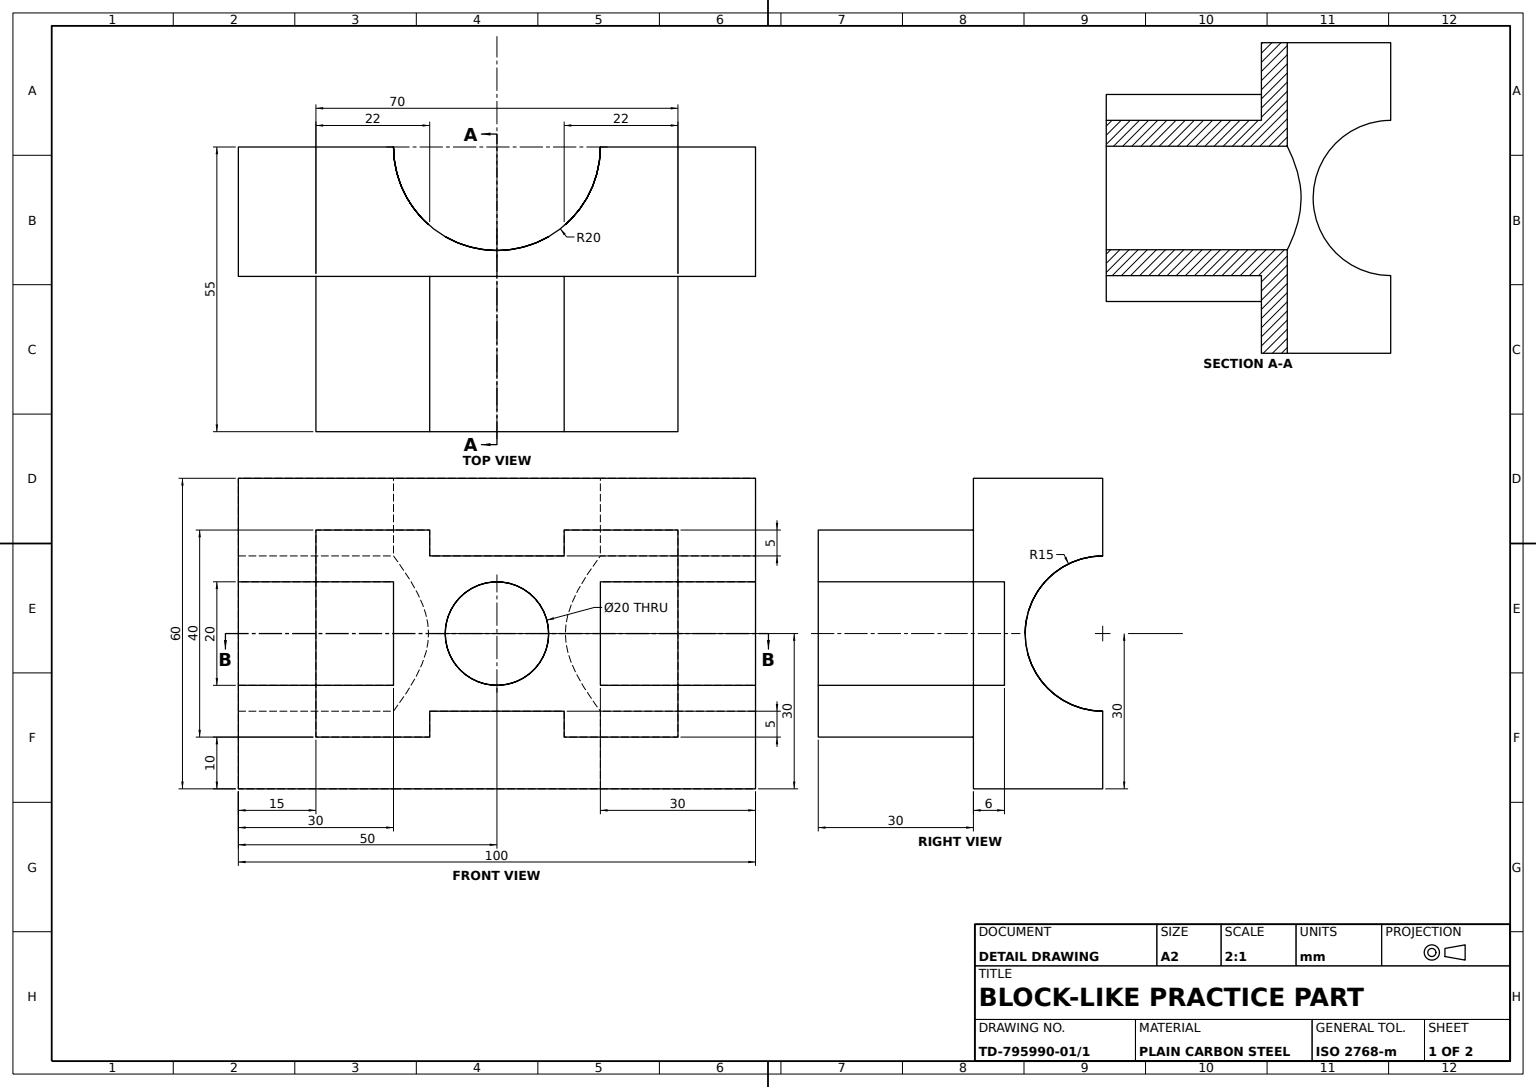
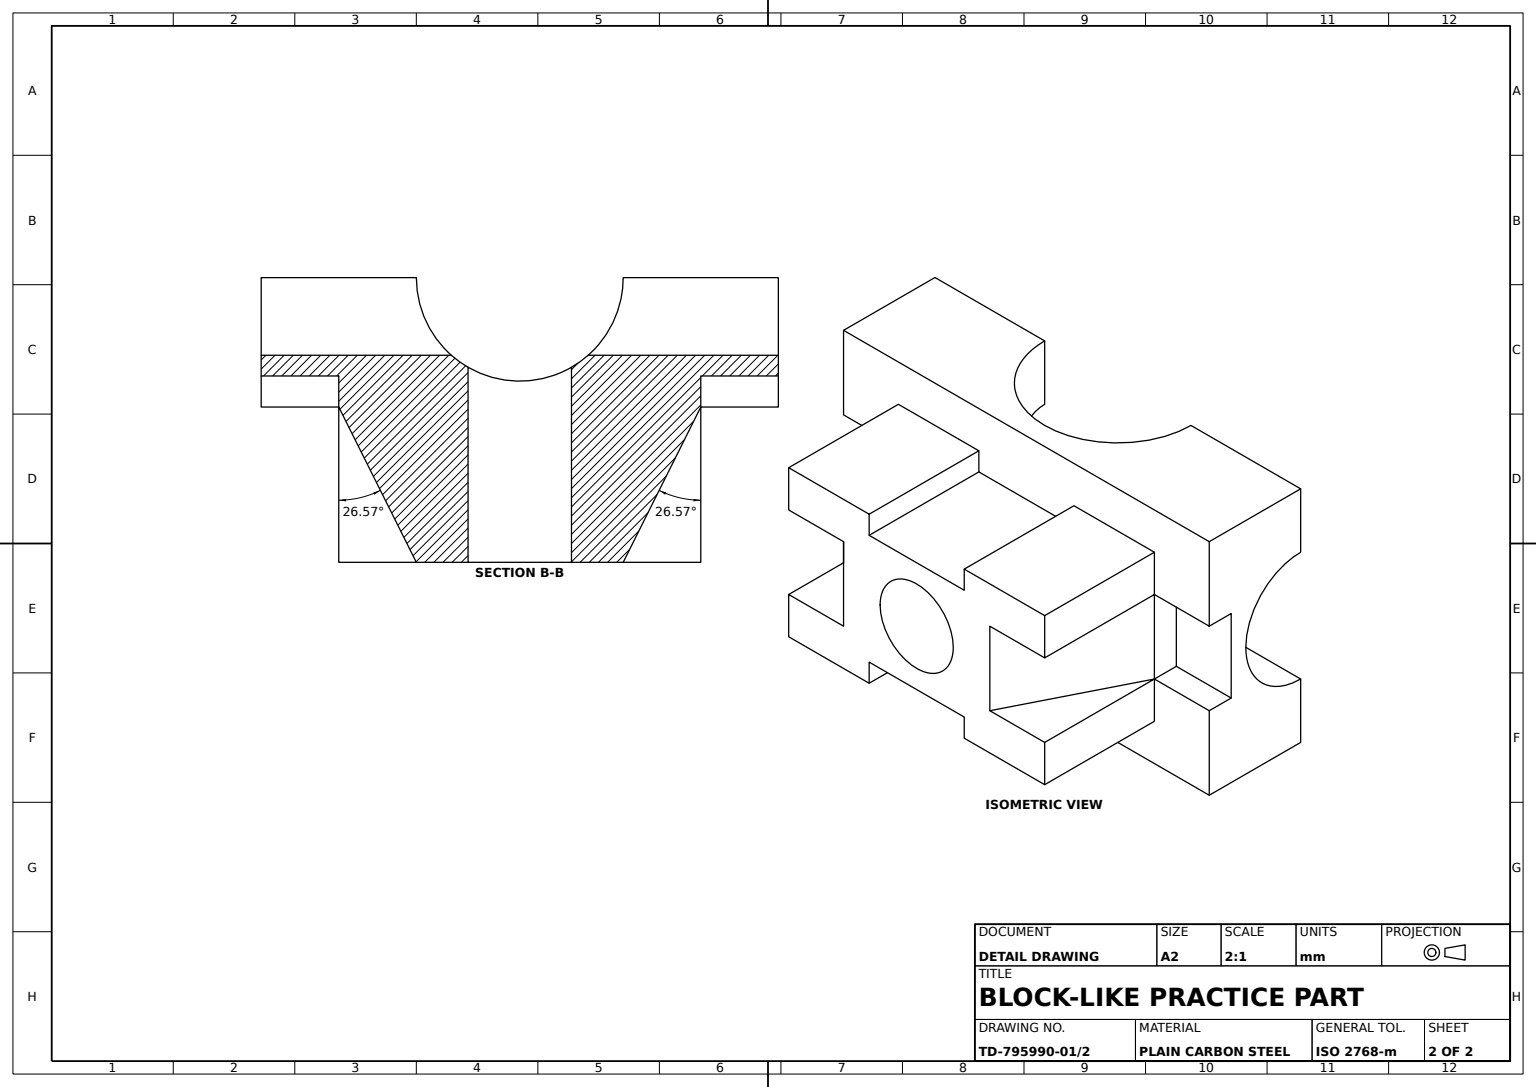
from build123d import *

# Parameters (mm, degrees)
BASE_PLATE_SKETCH_W        = 100
BASE_PLATE_SKETCH_H        = 60
BASE_PLATE_100X60X25_DEPTH = 25
T_BLOCK_SKETCH_W           = 70
T_BLOCK_SKETCH_H           = 40
T_BLOCK_70X40X30_DEPTH     = 30
SLOT_15X20_SKETCH_W        = 15
SLOT_15X20_SKETCH_H        = 20
SLOT_15X20_DEPTH_6_DEPTH   = 6
SECOND_SLOT_SKETCH_W       = 15
SECOND_SLOT_SKETCH_H       = 20
SECOND_SLOT_DEPTH_6_DEPTH  = 6
SIDE_ARC_NOTCH_DEPTH       = 60
END_ARC_NOTCH_DEPTH        = 100
BLOCK_RECESS_A_SKETCH_W    = 26
BLOCK_RECESS_A_SKETCH_H    = 5
BLOCK_RECESS_A_DEPTH       = 30
BLOCK_RECESS_B_SKETCH_W    = 26
BLOCK_RECESS_B_SKETCH_H    = 5
BLOCK_RECESS_B_DEPTH       = 30
CROSS_HOLE_SKETCH_R        = 10
CROSS_HOLE_DEPTH           = 55
WEDGE_CUT_A_DEPTH          = 30
WEDGE_FILL_A_DEPTH         = 10
WEDGE_CUT_B_DEPTH          = 30
WEDGE_FILL_B_DEPTH         = 10


with BuildPart() as part:
    # Base Plate Sketch → Base Plate 100x60x25 (new body)
    with BuildSketch(Plane.XY):
        with Locations((50, -30)):
            Rectangle(BASE_PLATE_SKETCH_W, BASE_PLATE_SKETCH_H)
    extrude(amount=BASE_PLATE_100X60X25_DEPTH)

    # T-Block Sketch → T-Block 70x40x30 (add)
    with BuildSketch(Plane.XY.offset(25)):
        with Locations((50, -30)):
            Rectangle(T_BLOCK_SKETCH_W, T_BLOCK_SKETCH_H)
    extrude(amount=T_BLOCK_70X40X30_DEPTH)

    # Slot 15x20 Sketch → Slot 15x20 Depth 6 (cut)
    with BuildSketch(Plane.XY.offset(25)):
        with Locations((7.5, -30)):
            Rectangle(SLOT_15X20_SKETCH_W, SLOT_15X20_SKETCH_H)
    extrude(amount=-SLOT_15X20_DEPTH_6_DEPTH, mode=Mode.SUBTRACT)

    # Second Slot Sketch → Second Slot Depth 6 (cut)
    with BuildSketch(Plane.XY.offset(25)):
        with Locations((92.5, -30)):
            Rectangle(SECOND_SLOT_SKETCH_W, SECOND_SLOT_SKETCH_H)
    extrude(amount=-SECOND_SLOT_DEPTH_6_DEPTH, mode=Mode.SUBTRACT)

    # Side Arc Notch Sketch → Side Arc Notch (cut)
    with BuildSketch(Plane.XZ.offset(60)):
        with BuildLine():
            Line((30, 0), (70, 0))
            ThreePointArc((70, 0), (50, 20), (30, 0))
        make_face()
    extrude(amount=-SIDE_ARC_NOTCH_DEPTH, mode=Mode.SUBTRACT)

    # End Arc Notch Sketch → End Arc Notch (cut)
    with BuildSketch(Plane.ZY):
        with BuildLine():
            Line((0, -15), (0, -45))
            ThreePointArc((0, -45), (15, -30), (0, -15))
        make_face()
    extrude(amount=-END_ARC_NOTCH_DEPTH, mode=Mode.SUBTRACT)

    # Block Recess A Sketch → Block Recess A (cut)
    with BuildSketch(Plane.XY.offset(55)):
        with Locations((50, -12.5)):
            Rectangle(BLOCK_RECESS_A_SKETCH_W, BLOCK_RECESS_A_SKETCH_H)
    extrude(amount=-BLOCK_RECESS_A_DEPTH, mode=Mode.SUBTRACT)

    # Block Recess B Sketch → Block Recess B (cut)
    with BuildSketch(Plane.XY.offset(55)):
        with Locations((50, -47.5)):
            Rectangle(BLOCK_RECESS_B_SKETCH_W, BLOCK_RECESS_B_SKETCH_H)
    extrude(amount=-BLOCK_RECESS_B_DEPTH, mode=Mode.SUBTRACT)

    # Cross Hole Sketch → Cross Hole (cut)
    with BuildSketch(Plane.XY.offset(55)):
        with Locations((50, -30)):
            Circle(CROSS_HOLE_SKETCH_R)
    extrude(amount=-CROSS_HOLE_DEPTH, mode=Mode.SUBTRACT)

    # Wedge Cut A Sketch → Wedge Cut A (cut)
    with BuildSketch(Plane.XZ.offset(50)):
        Polygon((15, 55), (30, 55), (15, 25), align=None)
    extrude(amount=-WEDGE_CUT_A_DEPTH, mode=Mode.SUBTRACT)

    # Wedge Fill A Sketch → Wedge Fill A (add)
    with BuildSketch(Plane.XZ.offset(50)):
        Polygon((15, 25), (15, 55), (30, 55), align=None)
    extrude(amount=-WEDGE_FILL_A_DEPTH)

    # Wedge Cut B Sketch → Wedge Cut B (cut)
    with BuildSketch(Plane.XZ.offset(50)):
        Polygon((85, 55), (70, 55), (85, 25), align=None)
    extrude(amount=-WEDGE_CUT_B_DEPTH, mode=Mode.SUBTRACT)

    # Wedge Fill B Sketch → Wedge Fill B (add)
    with BuildSketch(Plane.XZ.offset(50)):
        Polygon((70, 55), (85, 55), (85, 25), align=None)
    extrude(amount=-WEDGE_FILL_B_DEPTH)


solid = part.part
